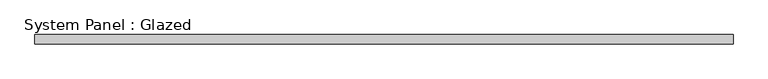
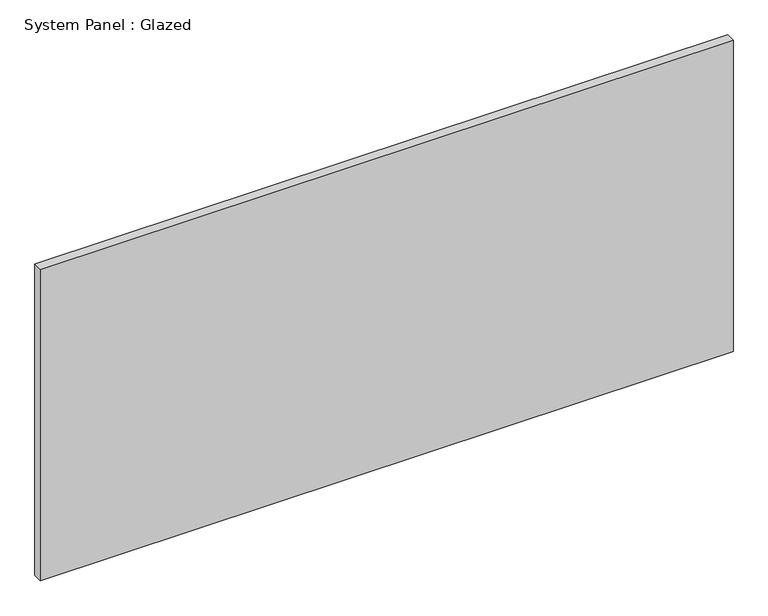
"""IFC4 building model written with IfcOpenShell, lengths in millimetres: plate geometry, System Panel : Glazed."""

from ifc_helpers import new_model, si_unit, origin, origin_with_axes, place, context, project, spatial, polyline, outline, extrude, source, transform, mapped, element, save


def system_panel_glazed_090522f0(model_context):
    return source(origin(), model_context, "Body", "SweptSolid", [
        extrude(outline(polyline([(967.3166667, 19.05), (-967.3166667, 19.05), (-967.3166667, 44.45), (967.3166667, 44.45), (967.3166667, 19.05)])), origin_with_axes(), (0.0, 0.0, 1.0), 919.5943516),
    ])


if __name__ == "__main__":
    model = new_model("IFC4")
    model_context = context("Model", 3, world=origin())
    ifc_project = project(units=[si_unit("LENGTHUNIT", "METRE", prefix="MILLI")], contexts=[model_context])
    site = spatial("IfcSite", under=ifc_project)
    building = spatial("IfcBuilding", under=site)
    placement = place(None, origin())
    system_panel_glazed_shape = system_panel_glazed_090522f0(model_context)
    element("IfcPlate", 1, ObjectType="System Panel : Glazed", at=placement, inside=building, context=model_context, shape_type="MappedRepresentation", body=[
        mapped(system_panel_glazed_shape, transform((0.0, 0.0, 0.0), x_axis=(1.0, 0.0, 0.0), y_axis=(0.0, 1.0, 0.0), z_axis=(0.0, 0.0, 1.0))),
    ])
    save(model, "model.ifc")

# Revit data of these elements
# Type "System Panel : Glazed"
#   Construction Type Id = "GSP4R"
#   Analytic Construction = "1/8 in Pilkington single glazing"
#   Visual Light Transmittance = 0.9
#   Solar Heat Gain Coefficient = 0.86
#   Heat Transfer Coefficient (U) = 1.18115 BTU/(h·ft²·°F)
#   Define Thermal Properties by = 1
# Element 1 (IfcPlate, "System Panel : Glazed")
#   Materials on its faces: "Glass"
# Materials
#   "Glass": class "Glass", colour RGB 0 128 192, transparency 0.75, Description = "Soda Lime Glass", Cost = 0
